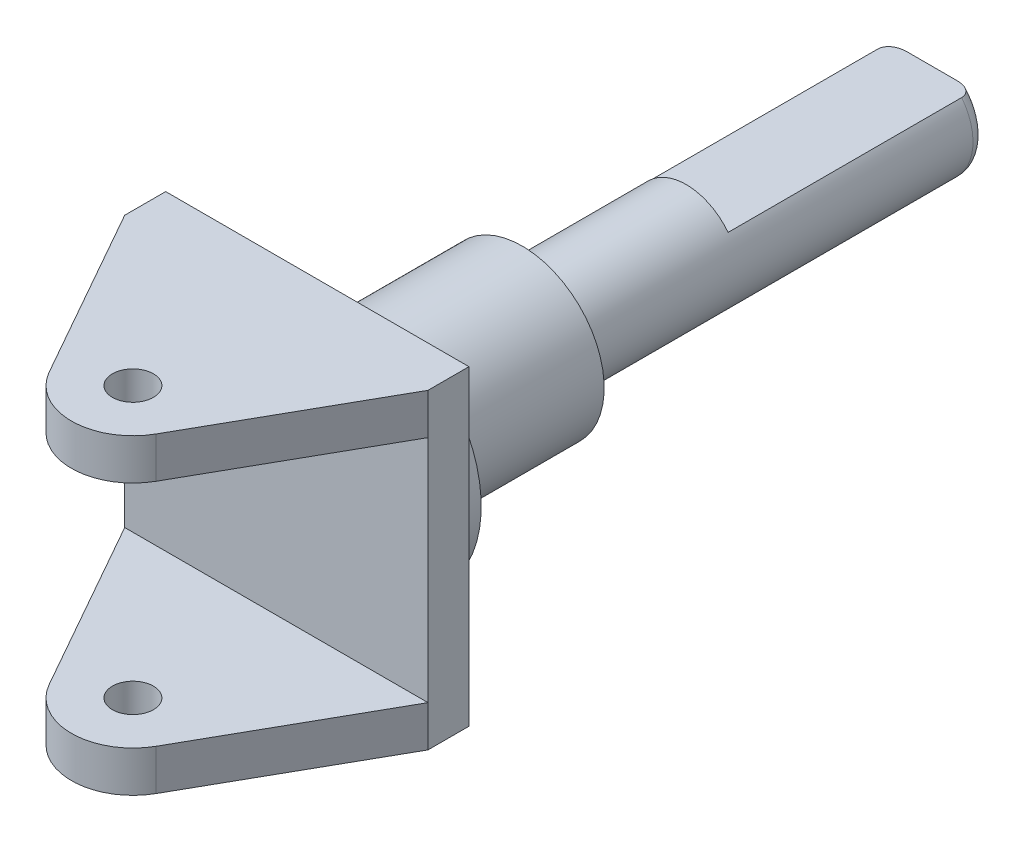
ISO-10303-21;
HEADER;
FILE_DESCRIPTION(('STEP AP214'),'2;1');
FILE_NAME('part.step','',(''),(''),'','','');
FILE_SCHEMA(('AUTOMOTIVE_DESIGN { 1 0 10303 214 1 1 1 1 }'));
ENDSEC;
DATA;
#1=APPLICATION_CONTEXT('core data for automotive mechanical design processes');
#2=APPLICATION_PROTOCOL_DEFINITION('international standard','automotive_design',2000,#1);
#3=PRODUCT_CONTEXT('',#1,'mechanical');
#4=PRODUCT('Part','Part','',(#3));
#5=PRODUCT_RELATED_PRODUCT_CATEGORY('part','',(#4));
#6=PRODUCT_DEFINITION_FORMATION('','',#4);
#7=PRODUCT_DEFINITION_CONTEXT('part definition',#1,'design');
#8=PRODUCT_DEFINITION('design','',#6,#7);
#9=PRODUCT_DEFINITION_SHAPE('','',#8);
#10=(LENGTH_UNIT() NAMED_UNIT(*) SI_UNIT(.MILLI.,.METRE.));
#11=(NAMED_UNIT(*) PLANE_ANGLE_UNIT() SI_UNIT($,.RADIAN.));
#12=(NAMED_UNIT(*) SI_UNIT($,.STERADIAN.) SOLID_ANGLE_UNIT());
#13=UNCERTAINTY_MEASURE_WITH_UNIT(LENGTH_MEASURE(1.E-05),#10,'distance_accuracy_value','');
#14=(GEOMETRIC_REPRESENTATION_CONTEXT(3) GLOBAL_UNCERTAINTY_ASSIGNED_CONTEXT((#13)) GLOBAL_UNIT_ASSIGNED_CONTEXT((#10,
#11,#12)) REPRESENTATION_CONTEXT('',''));
#15=CARTESIAN_POINT('',(0.,0.,0.));
#16=DIRECTION('',(0.,0.,1.));
#17=DIRECTION('',(1.,0.,0.));
#18=AXIS2_PLACEMENT_3D('',#15,#16,#17);
#19=CARTESIAN_POINT('',(0.,0.,10.));
#20=DIRECTION('',(0.,0.,-1.));
#21=DIRECTION('',(-1.,0.,0.));
#22=AXIS2_PLACEMENT_3D('',#19,#20,#21);
#23=PLANE('',#22);
#24=DIRECTION('',(0.,-1.,0.));
#25=VECTOR('',#24,1.);
#26=CARTESIAN_POINT('',(-37.,-38.,10.));
#27=LINE('',#26,#25);
#28=CARTESIAN_POINT('',(-37.,28.,10.));
#29=VERTEX_POINT('',#28);
#30=CARTESIAN_POINT('',(-37.,-28.,10.));
#31=VERTEX_POINT('',#30);
#32=EDGE_CURVE('E290',#29,#31,#27,.T.);
#33=ORIENTED_EDGE('',*,*,#32,.T.);
#34=DIRECTION('',(1.,0.,0.));
#35=VECTOR('',#34,1.);
#36=CARTESIAN_POINT('',(-37.,-28.,10.));
#37=LINE('',#36,#35);
#38=CARTESIAN_POINT('',(37.,-28.,10.));
#39=VERTEX_POINT('',#38);
#40=EDGE_CURVE('E224',#31,#39,#37,.T.);
#41=ORIENTED_EDGE('',*,*,#40,.T.);
#42=DIRECTION('',(0.,1.,0.));
#43=VECTOR('',#42,1.);
#44=CARTESIAN_POINT('',(37.,-38.,10.));
#45=LINE('',#44,#43);
#46=CARTESIAN_POINT('',(37.,28.,10.));
#47=VERTEX_POINT('',#46);
#48=EDGE_CURVE('E288',#39,#47,#45,.T.);
#49=ORIENTED_EDGE('',*,*,#48,.T.);
#50=DIRECTION('',(1.,0.,0.));
#51=VECTOR('',#50,1.);
#52=CARTESIAN_POINT('',(0.,28.,10.));
#53=LINE('',#52,#51);
#54=EDGE_CURVE('E263',#29,#47,#53,.T.);
#55=ORIENTED_EDGE('',*,*,#54,.F.);
#56=EDGE_LOOP('',(#33,#41,#49,#55));
#57=FACE_BOUND('',#56,.T.);
#58=ADVANCED_FACE('F41',(#57),#23,.F.);
#59=CARTESIAN_POINT('',(37.,-38.,10.));
#60=DIRECTION('',(-1.,0.,0.));
#61=DIRECTION('',(0.,0.,1.));
#62=AXIS2_PLACEMENT_3D('',#59,#60,#61);
#63=PLANE('',#62);
#64=DIRECTION('',(0.,1.,0.));
#65=VECTOR('',#64,1.);
#66=CARTESIAN_POINT('',(37.,-38.,0.));
#67=LINE('',#66,#65);
#68=CARTESIAN_POINT('',(37.,-38.,0.));
#69=VERTEX_POINT('',#68);
#70=CARTESIAN_POINT('',(37.,38.,0.));
#71=VERTEX_POINT('',#70);
#72=EDGE_CURVE('E278',#69,#71,#67,.T.);
#73=ORIENTED_EDGE('',*,*,#72,.T.);
#74=DIRECTION('',(0.,0.,-1.));
#75=VECTOR('',#74,1.);
#76=CARTESIAN_POINT('',(37.,38.,10.));
#77=LINE('',#76,#75);
#78=CARTESIAN_POINT('',(37.,38.,10.));
#79=VERTEX_POINT('',#78);
#80=EDGE_CURVE('E190',#79,#71,#77,.T.);
#81=ORIENTED_EDGE('',*,*,#80,.F.);
#82=DIRECTION('',(0.,1.,0.));
#83=VECTOR('',#82,1.);
#84=CARTESIAN_POINT('',(37.,28.,10.));
#85=LINE('',#84,#83);
#86=EDGE_CURVE('E280',#47,#79,#85,.T.);
#87=ORIENTED_EDGE('',*,*,#86,.F.);
#88=ORIENTED_EDGE('',*,*,#48,.F.);
#89=CARTESIAN_POINT('',(37.,-38.,10.));
#90=VERTEX_POINT('',#89);
#91=EDGE_CURVE('E282',#90,#39,#45,.T.);
#92=ORIENTED_EDGE('',*,*,#91,.F.);
#93=DIRECTION('',(0.,0.,-1.));
#94=VECTOR('',#93,1.);
#95=CARTESIAN_POINT('',(37.,-38.,10.));
#96=LINE('',#95,#94);
#97=EDGE_CURVE('E295',#90,#69,#96,.T.);
#98=ORIENTED_EDGE('',*,*,#97,.T.);
#99=EDGE_LOOP('',(#73,#81,#87,#88,#92,#98));
#100=FACE_BOUND('',#99,.T.);
#101=ADVANCED_FACE('F403',(#100),#63,.F.);
#102=CARTESIAN_POINT('',(-37.,38.,10.));
#103=DIRECTION('',(0.,-1.,0.));
#104=DIRECTION('',(0.,0.,-1.));
#105=AXIS2_PLACEMENT_3D('',#102,#103,#104);
#106=PLANE('',#105);
#107=DIRECTION('',(-1.,0.,0.));
#108=VECTOR('',#107,1.);
#109=CARTESIAN_POINT('',(-37.,38.,0.));
#110=LINE('',#109,#108);
#111=CARTESIAN_POINT('',(-37.,38.,0.));
#112=VERTEX_POINT('',#111);
#113=EDGE_CURVE('E293',#71,#112,#110,.T.);
#114=ORIENTED_EDGE('',*,*,#113,.T.);
#115=DIRECTION('',(0.,0.,-1.));
#116=VECTOR('',#115,1.);
#117=CARTESIAN_POINT('',(-37.,38.,10.));
#118=LINE('',#117,#116);
#119=CARTESIAN_POINT('',(-37.,38.,10.));
#120=VERTEX_POINT('',#119);
#121=EDGE_CURVE('E308',#120,#112,#118,.T.);
#122=ORIENTED_EDGE('',*,*,#121,.F.);
#123=DIRECTION('',(0.491857302042567,0.,0.870675826256482));
#124=VECTOR('',#123,1.);
#125=CARTESIAN_POINT('',(-32.331309222376,38.,18.2644217814052));
#126=LINE('',#125,#124);
#127=CARTESIAN_POINT('',(-13.0601373938472,38.,52.3778595306385));
#128=VERTEX_POINT('',#127);
#129=EDGE_CURVE('E267',#120,#128,#126,.T.);
#130=ORIENTED_EDGE('',*,*,#129,.T.);
#131=CARTESIAN_POINT('',(0.,38.,45.));
#132=DIRECTION('',(0.,1.,0.));
#133=DIRECTION('',(0.,0.,1.));
#134=AXIS2_PLACEMENT_3D('',#131,#132,#133);
#135=CIRCLE('',#134,15.);
#136=CARTESIAN_POINT('',(13.0601373938472,38.,52.3778595306385));
#137=VERTEX_POINT('',#136);
#138=EDGE_CURVE('E275',#128,#137,#135,.T.);
#139=ORIENTED_EDGE('',*,*,#138,.T.);
#140=DIRECTION('',(0.491857302042567,0.,-0.870675826256482));
#141=VECTOR('',#140,1.);
#142=CARTESIAN_POINT('',(32.331309222376,38.,18.2644217814052));
#143=LINE('',#142,#141);
#144=EDGE_CURVE('E255',#137,#79,#143,.T.);
#145=ORIENTED_EDGE('',*,*,#144,.T.);
#146=ORIENTED_EDGE('',*,*,#80,.T.);
#147=EDGE_LOOP('',(#114,#122,#130,#139,#145,#146));
#148=FACE_BOUND('',#147,.T.);
#149=CARTESIAN_POINT('',(0.,38.,45.));
#150=DIRECTION('',(0.,1.,0.));
#151=DIRECTION('',(0.,0.,1.));
#152=AXIS2_PLACEMENT_3D('',#149,#150,#151);
#153=CIRCLE('',#152,5.);
#154=CARTESIAN_POINT('',(0.,38.,50.));
#155=VERTEX_POINT('',#154);
#156=EDGE_CURVE('E247',#155,#155,#153,.T.);
#157=ORIENTED_EDGE('',*,*,#156,.F.);
#158=EDGE_LOOP('',(#157));
#159=FACE_BOUND('',#158,.T.);
#160=ADVANCED_FACE('F417',(#148,#159),#106,.F.);
#161=CARTESIAN_POINT('',(-37.,-38.,10.));
#162=DIRECTION('',(1.,0.,0.));
#163=DIRECTION('',(0.,0.,-1.));
#164=AXIS2_PLACEMENT_3D('',#161,#162,#163);
#165=PLANE('',#164);
#166=DIRECTION('',(0.,-1.,0.));
#167=VECTOR('',#166,1.);
#168=CARTESIAN_POINT('',(-37.,-38.,0.));
#169=LINE('',#168,#167);
#170=CARTESIAN_POINT('',(-37.,-38.,0.));
#171=VERTEX_POINT('',#170);
#172=EDGE_CURVE('E300',#112,#171,#169,.T.);
#173=ORIENTED_EDGE('',*,*,#172,.T.);
#174=DIRECTION('',(0.,0.,-1.));
#175=VECTOR('',#174,1.);
#176=CARTESIAN_POINT('',(-37.,-38.,10.));
#177=LINE('',#176,#175);
#178=CARTESIAN_POINT('',(-37.,-38.,10.));
#179=VERTEX_POINT('',#178);
#180=EDGE_CURVE('E303',#179,#171,#177,.T.);
#181=ORIENTED_EDGE('',*,*,#180,.F.);
#182=DIRECTION('',(0.,-1.,0.));
#183=VECTOR('',#182,1.);
#184=CARTESIAN_POINT('',(-37.,-28.,10.));
#185=LINE('',#184,#183);
#186=EDGE_CURVE('E241',#31,#179,#185,.T.);
#187=ORIENTED_EDGE('',*,*,#186,.F.);
#188=ORIENTED_EDGE('',*,*,#32,.F.);
#189=EDGE_CURVE('E289',#120,#29,#27,.T.);
#190=ORIENTED_EDGE('',*,*,#189,.F.);
#191=ORIENTED_EDGE('',*,*,#121,.T.);
#192=EDGE_LOOP('',(#173,#181,#187,#188,#190,#191));
#193=FACE_BOUND('',#192,.T.);
#194=ADVANCED_FACE('F413',(#193),#165,.F.);
#195=CARTESIAN_POINT('',(-37.,-38.,10.));
#196=DIRECTION('',(0.,1.,0.));
#197=DIRECTION('',(0.,0.,1.));
#198=AXIS2_PLACEMENT_3D('',#195,#196,#197);
#199=PLANE('',#198);
#200=DIRECTION('',(1.,0.,0.));
#201=VECTOR('',#200,1.);
#202=CARTESIAN_POINT('',(-37.,-38.,0.));
#203=LINE('',#202,#201);
#204=EDGE_CURVE('E297',#171,#69,#203,.T.);
#205=ORIENTED_EDGE('',*,*,#204,.T.);
#206=ORIENTED_EDGE('',*,*,#97,.F.);
#207=DIRECTION('',(-0.491857302042567,0.,0.870675826256482));
#208=VECTOR('',#207,1.);
#209=CARTESIAN_POINT('',(37.,-38.,10.));
#210=LINE('',#209,#208);
#211=CARTESIAN_POINT('',(13.0601373938472,-38.,52.3778595306385));
#212=VERTEX_POINT('',#211);
#213=EDGE_CURVE('E219',#90,#212,#210,.T.);
#214=ORIENTED_EDGE('',*,*,#213,.T.);
#215=CARTESIAN_POINT('',(0.,-38.,44.9999999999996));
#216=DIRECTION('',(0.,-1.,0.));
#217=DIRECTION('',(0.,0.,1.));
#218=AXIS2_PLACEMENT_3D('',#215,#216,#217);
#219=CIRCLE('',#218,15.0000000000002);
#220=CARTESIAN_POINT('',(-13.0601373938472,-38.,52.3778595306385));
#221=VERTEX_POINT('',#220);
#222=EDGE_CURVE('E236',#212,#221,#219,.T.);
#223=ORIENTED_EDGE('',*,*,#222,.T.);
#224=DIRECTION('',(-0.491857302042567,0.,-0.870675826256482));
#225=VECTOR('',#224,1.);
#226=CARTESIAN_POINT('',(-37.,-38.,10.));
#227=LINE('',#226,#225);
#228=EDGE_CURVE('E228',#221,#179,#227,.T.);
#229=ORIENTED_EDGE('',*,*,#228,.T.);
#230=ORIENTED_EDGE('',*,*,#180,.T.);
#231=EDGE_LOOP('',(#205,#206,#214,#223,#229,#230));
#232=FACE_BOUND('',#231,.T.);
#233=CARTESIAN_POINT('',(0.,-38.,44.9999999999996));
#234=DIRECTION('',(0.,-1.,0.));
#235=DIRECTION('',(0.,0.,-1.));
#236=AXIS2_PLACEMENT_3D('',#233,#234,#235);
#237=CIRCLE('',#236,4.9999999999998);
#238=CARTESIAN_POINT('',(0.,-38.,39.9999999999998));
#239=VERTEX_POINT('',#238);
#240=EDGE_CURVE('E216',#239,#239,#237,.T.);
#241=ORIENTED_EDGE('',*,*,#240,.F.);
#242=EDGE_LOOP('',(#241));
#243=FACE_BOUND('',#242,.T.);
#244=ADVANCED_FACE('F407',(#232,#243),#199,.F.);
#245=CARTESIAN_POINT('',(0.,0.,0.));
#246=DIRECTION('',(0.,0.,-1.));
#247=DIRECTION('',(-1.,0.,0.));
#248=AXIS2_PLACEMENT_3D('',#245,#246,#247);
#249=PLANE('',#248);
#250=CARTESIAN_POINT('',(0.,0.,0.));
#251=DIRECTION('',(0.,0.,-1.));
#252=DIRECTION('',(-1.,0.,0.));
#253=AXIS2_PLACEMENT_3D('',#250,#251,#252);
#254=CIRCLE('',#253,30.);
#255=CARTESIAN_POINT('',(-19.9214744270855,-22.4306677709555,0.));
#256=VERTEX_POINT('',#255);
#257=CARTESIAN_POINT('',(-19.9214744270848,22.430667770956,0.));
#258=VERTEX_POINT('',#257);
#259=EDGE_CURVE('E184',#256,#258,#254,.T.);
#260=ORIENTED_EDGE('',*,*,#259,.F.);
#261=DIRECTION('',(-0.999883722331186,-0.0152493218580814,0.));
#262=VECTOR('',#261,1.);
#263=CARTESIAN_POINT('',(0.337380123403688,-22.1216980511602,0.));
#264=LINE('',#263,#262);
#265=CARTESIAN_POINT('',(20.5962346738928,-21.812728331365,0.));
#266=VERTEX_POINT('',#265);
#267=EDGE_CURVE('E192',#266,#256,#264,.T.);
#268=ORIENTED_EDGE('',*,*,#267,.F.);
#269=CARTESIAN_POINT('',(0.,0.,0.));
#270=DIRECTION('',(0.,0.,-1.));
#271=DIRECTION('',(-1.,0.,0.));
#272=AXIS2_PLACEMENT_3D('',#269,#270,#271);
#273=CIRCLE('',#272,30.);
#274=CARTESIAN_POINT('',(20.5962346738934,21.8127283313644,0.));
#275=VERTEX_POINT('',#274);
#276=EDGE_CURVE('E201',#275,#266,#273,.T.);
#277=ORIENTED_EDGE('',*,*,#276,.F.);
#278=DIRECTION('',(-0.999883722331186,0.0152493218581099,0.));
#279=VECTOR('',#278,1.);
#280=CARTESIAN_POINT('',(0.337380123404318,22.1216980511602,0.));
#281=LINE('',#280,#279);
#282=EDGE_CURVE('E199',#275,#258,#281,.T.);
#283=ORIENTED_EDGE('',*,*,#282,.T.);
#284=EDGE_LOOP('',(#260,#268,#277,#283));
#285=FACE_BOUND('',#284,.T.);
#286=ORIENTED_EDGE('',*,*,#72,.F.);
#287=ORIENTED_EDGE('',*,*,#204,.F.);
#288=ORIENTED_EDGE('',*,*,#172,.F.);
#289=ORIENTED_EDGE('',*,*,#113,.F.);
#290=EDGE_LOOP('',(#286,#287,#288,#289));
#291=FACE_BOUND('',#290,.T.);
#292=ADVANCED_FACE('F398',(#285,#291),#249,.T.);
#293=CARTESIAN_POINT('',(-32.331309222376,28.,18.2644217814052));
#294=DIRECTION('',(-0.870675826256482,0.,0.491857302042566));
#295=DIRECTION('',(0.491857302042566,0.,0.870675826256482));
#296=AXIS2_PLACEMENT_3D('',#293,#294,#295);
#297=PLANE('',#296);
#298=ORIENTED_EDGE('',*,*,#129,.F.);
#299=ORIENTED_EDGE('',*,*,#189,.T.);
#300=DIRECTION('',(0.491857302042567,0.,0.870675826256482));
#301=VECTOR('',#300,1.);
#302=CARTESIAN_POINT('',(-32.331309222376,28.,18.2644217814052));
#303=LINE('',#302,#301);
#304=CARTESIAN_POINT('',(-13.0601373938472,28.,52.3778595306385));
#305=VERTEX_POINT('',#304);
#306=EDGE_CURVE('E251',#29,#305,#303,.T.);
#307=ORIENTED_EDGE('',*,*,#306,.T.);
#308=DIRECTION('',(0.,1.,0.));
#309=VECTOR('',#308,1.);
#310=CARTESIAN_POINT('',(-13.0601373938472,28.,52.3778595306385));
#311=LINE('',#310,#309);
#312=EDGE_CURVE('E266',#305,#128,#311,.T.);
#313=ORIENTED_EDGE('',*,*,#312,.T.);
#314=EDGE_LOOP('',(#298,#299,#307,#313));
#315=FACE_BOUND('',#314,.T.);
#316=ADVANCED_FACE('F393',(#315),#297,.T.);
#317=CARTESIAN_POINT('',(32.331309222376,28.,18.2644217814052));
#318=DIRECTION('',(0.870675826256482,0.,0.491857302042567));
#319=DIRECTION('',(0.491857302042567,0.,-0.870675826256482));
#320=AXIS2_PLACEMENT_3D('',#317,#318,#319);
#321=PLANE('',#320);
#322=ORIENTED_EDGE('',*,*,#144,.F.);
#323=DIRECTION('',(0.,1.,0.));
#324=VECTOR('',#323,1.);
#325=CARTESIAN_POINT('',(13.0601373938472,28.,52.3778595306385));
#326=LINE('',#325,#324);
#327=CARTESIAN_POINT('',(13.0601373938472,28.,52.3778595306385));
#328=VERTEX_POINT('',#327);
#329=EDGE_CURVE('E283',#328,#137,#326,.T.);
#330=ORIENTED_EDGE('',*,*,#329,.F.);
#331=DIRECTION('',(0.491857302042567,0.,-0.870675826256482));
#332=VECTOR('',#331,1.);
#333=CARTESIAN_POINT('',(32.331309222376,28.,18.2644217814052));
#334=LINE('',#333,#332);
#335=EDGE_CURVE('E257',#328,#47,#334,.T.);
#336=ORIENTED_EDGE('',*,*,#335,.T.);
#337=ORIENTED_EDGE('',*,*,#86,.T.);
#338=EDGE_LOOP('',(#322,#330,#336,#337));
#339=FACE_BOUND('',#338,.T.);
#340=ADVANCED_FACE('F390',(#339),#321,.T.);
#341=CARTESIAN_POINT('',(0.,28.,45.));
#342=DIRECTION('',(0.,1.,0.));
#343=DIRECTION('',(0.,0.,1.));
#344=AXIS2_PLACEMENT_3D('',#341,#342,#343);
#345=CYLINDRICAL_SURFACE('',#344,5.);
#346=CARTESIAN_POINT('',(0.,28.,45.));
#347=DIRECTION('',(0.,1.,0.));
#348=DIRECTION('',(0.,0.,1.));
#349=AXIS2_PLACEMENT_3D('',#346,#347,#348);
#350=CIRCLE('',#349,5.);
#351=CARTESIAN_POINT('',(0.,28.,50.));
#352=VERTEX_POINT('',#351);
#353=EDGE_CURVE('E246',#352,#352,#350,.T.);
#354=ORIENTED_EDGE('',*,*,#353,.F.);
#355=EDGE_LOOP('',(#354));
#356=FACE_BOUND('',#355,.T.);
#357=ORIENTED_EDGE('',*,*,#156,.T.);
#358=EDGE_LOOP('',(#357));
#359=FACE_BOUND('',#358,.T.);
#360=ADVANCED_FACE('F388',(#356,#359),#345,.F.);
#361=CARTESIAN_POINT('',(0.,28.,45.));
#362=DIRECTION('',(0.,1.,0.));
#363=DIRECTION('',(0.,0.,1.));
#364=AXIS2_PLACEMENT_3D('',#361,#362,#363);
#365=CYLINDRICAL_SURFACE('',#364,15.);
#366=ORIENTED_EDGE('',*,*,#138,.F.);
#367=ORIENTED_EDGE('',*,*,#312,.F.);
#368=CARTESIAN_POINT('',(0.,28.,45.));
#369=DIRECTION('',(0.,1.,0.));
#370=DIRECTION('',(0.,0.,1.));
#371=AXIS2_PLACEMENT_3D('',#368,#369,#370);
#372=CIRCLE('',#371,15.);
#373=EDGE_CURVE('E260',#305,#328,#372,.T.);
#374=ORIENTED_EDGE('',*,*,#373,.T.);
#375=ORIENTED_EDGE('',*,*,#329,.T.);
#376=EDGE_LOOP('',(#366,#367,#374,#375));
#377=FACE_BOUND('',#376,.T.);
#378=ADVANCED_FACE('F384',(#377),#365,.T.);
#379=CARTESIAN_POINT('',(0.,28.,0.));
#380=DIRECTION('',(0.,1.,0.));
#381=DIRECTION('',(0.,0.,1.));
#382=AXIS2_PLACEMENT_3D('',#379,#380,#381);
#383=PLANE('',#382);
#384=ORIENTED_EDGE('',*,*,#353,.T.);
#385=EDGE_LOOP('',(#384));
#386=FACE_BOUND('',#385,.T.);
#387=ORIENTED_EDGE('',*,*,#306,.F.);
#388=ORIENTED_EDGE('',*,*,#54,.T.);
#389=ORIENTED_EDGE('',*,*,#335,.F.);
#390=ORIENTED_EDGE('',*,*,#373,.F.);
#391=EDGE_LOOP('',(#387,#388,#389,#390));
#392=FACE_BOUND('',#391,.T.);
#393=ADVANCED_FACE('F374',(#386,#392),#383,.F.);
#394=CARTESIAN_POINT('',(-37.,-28.,10.));
#395=DIRECTION('',(-0.870675826256482,0.,0.491857302042567));
#396=DIRECTION('',(0.491857302042567,0.,0.870675826256482));
#397=AXIS2_PLACEMENT_3D('',#394,#395,#396);
#398=PLANE('',#397);
#399=ORIENTED_EDGE('',*,*,#228,.F.);
#400=DIRECTION('',(0.,-1.,0.));
#401=VECTOR('',#400,1.);
#402=CARTESIAN_POINT('',(-13.0601373938472,-28.,52.3778595306385));
#403=LINE('',#402,#401);
#404=CARTESIAN_POINT('',(-13.0601373938472,-28.,52.3778595306385));
#405=VERTEX_POINT('',#404);
#406=EDGE_CURVE('E250',#405,#221,#403,.T.);
#407=ORIENTED_EDGE('',*,*,#406,.F.);
#408=DIRECTION('',(-0.491857302042567,0.,-0.870675826256482));
#409=VECTOR('',#408,1.);
#410=CARTESIAN_POINT('',(-37.,-28.,10.));
#411=LINE('',#410,#409);
#412=EDGE_CURVE('E235',#405,#31,#411,.T.);
#413=ORIENTED_EDGE('',*,*,#412,.T.);
#414=ORIENTED_EDGE('',*,*,#186,.T.);
#415=EDGE_LOOP('',(#399,#407,#413,#414));
#416=FACE_BOUND('',#415,.T.);
#417=ADVANCED_FACE('F371',(#416),#398,.T.);
#418=CARTESIAN_POINT('',(0.,-28.,44.9999999999996));
#419=DIRECTION('',(0.,-1.,0.));
#420=DIRECTION('',(0.,0.,-1.));
#421=AXIS2_PLACEMENT_3D('',#418,#419,#420);
#422=CYLINDRICAL_SURFACE('',#421,15.0000000000002);
#423=ORIENTED_EDGE('',*,*,#222,.F.);
#424=DIRECTION('',(0.,-1.,0.));
#425=VECTOR('',#424,1.);
#426=CARTESIAN_POINT('',(13.0601373938472,-28.,52.3778595306385));
#427=LINE('',#426,#425);
#428=CARTESIAN_POINT('',(13.0601373938472,-28.,52.3778595306385));
#429=VERTEX_POINT('',#428);
#430=EDGE_CURVE('E231',#429,#212,#427,.T.);
#431=ORIENTED_EDGE('',*,*,#430,.F.);
#432=CARTESIAN_POINT('',(0.,-28.,44.9999999999996));
#433=DIRECTION('',(0.,-1.,0.));
#434=DIRECTION('',(0.,0.,1.));
#435=AXIS2_PLACEMENT_3D('',#432,#433,#434);
#436=CIRCLE('',#435,15.0000000000002);
#437=EDGE_CURVE('E227',#429,#405,#436,.T.);
#438=ORIENTED_EDGE('',*,*,#437,.T.);
#439=ORIENTED_EDGE('',*,*,#406,.T.);
#440=EDGE_LOOP('',(#423,#431,#438,#439));
#441=FACE_BOUND('',#440,.T.);
#442=ADVANCED_FACE('F372',(#441),#422,.T.);
#443=CARTESIAN_POINT('',(37.,-28.,10.));
#444=DIRECTION('',(0.870675826256482,0.,0.491857302042566));
#445=DIRECTION('',(0.491857302042566,0.,-0.870675826256482));
#446=AXIS2_PLACEMENT_3D('',#443,#444,#445);
#447=PLANE('',#446);
#448=ORIENTED_EDGE('',*,*,#213,.F.);
#449=ORIENTED_EDGE('',*,*,#91,.T.);
#450=DIRECTION('',(-0.491857302042567,0.,0.870675826256482));
#451=VECTOR('',#450,1.);
#452=CARTESIAN_POINT('',(37.,-28.,10.));
#453=LINE('',#452,#451);
#454=EDGE_CURVE('E223',#39,#429,#453,.T.);
#455=ORIENTED_EDGE('',*,*,#454,.T.);
#456=ORIENTED_EDGE('',*,*,#430,.T.);
#457=EDGE_LOOP('',(#448,#449,#455,#456));
#458=FACE_BOUND('',#457,.T.);
#459=ADVANCED_FACE('F369',(#458),#447,.T.);
#460=CARTESIAN_POINT('',(0.,-28.,44.9999999999996));
#461=DIRECTION('',(0.,1.,0.));
#462=DIRECTION('',(0.,0.,1.));
#463=AXIS2_PLACEMENT_3D('',#460,#461,#462);
#464=PLANE('',#463);
#465=CARTESIAN_POINT('',(0.,-28.,44.9999999999996));
#466=DIRECTION('',(0.,-1.,0.));
#467=DIRECTION('',(0.,0.,-1.));
#468=AXIS2_PLACEMENT_3D('',#465,#466,#467);
#469=CIRCLE('',#468,4.9999999999998);
#470=CARTESIAN_POINT('',(0.,-28.,39.9999999999998));
#471=VERTEX_POINT('',#470);
#472=EDGE_CURVE('E220',#471,#471,#469,.T.);
#473=ORIENTED_EDGE('',*,*,#472,.T.);
#474=EDGE_LOOP('',(#473));
#475=FACE_BOUND('',#474,.T.);
#476=ORIENTED_EDGE('',*,*,#40,.F.);
#477=ORIENTED_EDGE('',*,*,#412,.F.);
#478=ORIENTED_EDGE('',*,*,#437,.F.);
#479=ORIENTED_EDGE('',*,*,#454,.F.);
#480=EDGE_LOOP('',(#476,#477,#478,#479));
#481=FACE_BOUND('',#480,.T.);
#482=ADVANCED_FACE('F364',(#475,#481),#464,.T.);
#483=CARTESIAN_POINT('',(0.,-28.,44.9999999999996));
#484=DIRECTION('',(0.,-1.,0.));
#485=DIRECTION('',(0.,0.,-1.));
#486=AXIS2_PLACEMENT_3D('',#483,#484,#485);
#487=CYLINDRICAL_SURFACE('',#486,4.9999999999998);
#488=ORIENTED_EDGE('',*,*,#472,.F.);
#489=EDGE_LOOP('',(#488));
#490=FACE_BOUND('',#489,.T.);
#491=ORIENTED_EDGE('',*,*,#240,.T.);
#492=EDGE_LOOP('',(#491));
#493=FACE_BOUND('',#492,.T.);
#494=ADVANCED_FACE('F363',(#490,#493),#487,.F.);
#495=CARTESIAN_POINT('',(0.,0.,-10.));
#496=DIRECTION('',(0.,0.,1.));
#497=DIRECTION('',(1.,0.,0.));
#498=AXIS2_PLACEMENT_3D('',#495,#496,#497);
#499=CYLINDRICAL_SURFACE('',#498,30.);
#500=ORIENTED_EDGE('',*,*,#259,.T.);
#501=DIRECTION('',(0.,0.,1.));
#502=VECTOR('',#501,1.);
#503=CARTESIAN_POINT('',(-19.9214744270848,22.430667770956,-10.));
#504=LINE('',#503,#502);
#505=CARTESIAN_POINT('',(-19.9214744270848,22.430667770956,-10.));
#506=VERTEX_POINT('',#505);
#507=EDGE_CURVE('E213',#506,#258,#504,.T.);
#508=ORIENTED_EDGE('',*,*,#507,.F.);
#509=CARTESIAN_POINT('',(0.,0.,-10.));
#510=DIRECTION('',(0.,0.,-1.));
#511=DIRECTION('',(-1.,0.,0.));
#512=AXIS2_PLACEMENT_3D('',#509,#510,#511);
#513=CIRCLE('',#512,30.);
#514=CARTESIAN_POINT('',(-19.9214744270855,-22.4306677709555,-10.));
#515=VERTEX_POINT('',#514);
#516=EDGE_CURVE('E186',#515,#506,#513,.T.);
#517=ORIENTED_EDGE('',*,*,#516,.F.);
#518=DIRECTION('',(0.,0.,1.));
#519=VECTOR('',#518,1.);
#520=CARTESIAN_POINT('',(-19.9214744270855,-22.4306677709555,-10.));
#521=LINE('',#520,#519);
#522=EDGE_CURVE('E196',#515,#256,#521,.T.);
#523=ORIENTED_EDGE('',*,*,#522,.T.);
#524=EDGE_LOOP('',(#500,#508,#517,#523));
#525=FACE_BOUND('',#524,.T.);
#526=ADVANCED_FACE('F360',(#525),#499,.T.);
#527=CARTESIAN_POINT('',(0.337380123404318,22.1216980511602,-10.));
#528=DIRECTION('',(0.0152493218581099,0.999883722331186,0.));
#529=DIRECTION('',(-0.999883722331186,0.0152493218581099,0.));
#530=AXIS2_PLACEMENT_3D('',#527,#528,#529);
#531=PLANE('',#530);
#532=ORIENTED_EDGE('',*,*,#282,.F.);
#533=DIRECTION('',(0.,0.,1.));
#534=VECTOR('',#533,1.);
#535=CARTESIAN_POINT('',(20.5962346738934,21.8127283313644,-10.));
#536=LINE('',#535,#534);
#537=CARTESIAN_POINT('',(20.5962346738934,21.8127283313644,-10.));
#538=VERTEX_POINT('',#537);
#539=EDGE_CURVE('E211',#538,#275,#536,.T.);
#540=ORIENTED_EDGE('',*,*,#539,.F.);
#541=DIRECTION('',(-0.999883722331186,0.0152493218581099,0.));
#542=VECTOR('',#541,1.);
#543=CARTESIAN_POINT('',(0.337380123404318,22.1216980511602,-10.));
#544=LINE('',#543,#542);
#545=EDGE_CURVE('E189',#538,#506,#544,.T.);
#546=ORIENTED_EDGE('',*,*,#545,.T.);
#547=ORIENTED_EDGE('',*,*,#507,.T.);
#548=EDGE_LOOP('',(#532,#540,#546,#547));
#549=FACE_BOUND('',#548,.T.);
#550=ADVANCED_FACE('F351',(#549),#531,.T.);
#551=CARTESIAN_POINT('',(0.,0.,-10.));
#552=DIRECTION('',(0.,0.,1.));
#553=DIRECTION('',(1.,0.,0.));
#554=AXIS2_PLACEMENT_3D('',#551,#552,#553);
#555=CYLINDRICAL_SURFACE('',#554,30.);
#556=ORIENTED_EDGE('',*,*,#276,.T.);
#557=DIRECTION('',(0.,0.,1.));
#558=VECTOR('',#557,1.);
#559=CARTESIAN_POINT('',(20.5962346738928,-21.812728331365,-10.));
#560=LINE('',#559,#558);
#561=CARTESIAN_POINT('',(20.5962346738928,-21.812728331365,-10.));
#562=VERTEX_POINT('',#561);
#563=EDGE_CURVE('E208',#562,#266,#560,.T.);
#564=ORIENTED_EDGE('',*,*,#563,.F.);
#565=CARTESIAN_POINT('',(0.,0.,-10.));
#566=DIRECTION('',(0.,0.,-1.));
#567=DIRECTION('',(-1.,0.,0.));
#568=AXIS2_PLACEMENT_3D('',#565,#566,#567);
#569=CIRCLE('',#568,30.);
#570=EDGE_CURVE('E194',#538,#562,#569,.T.);
#571=ORIENTED_EDGE('',*,*,#570,.F.);
#572=ORIENTED_EDGE('',*,*,#539,.T.);
#573=EDGE_LOOP('',(#556,#564,#571,#572));
#574=FACE_BOUND('',#573,.T.);
#575=ADVANCED_FACE('F349',(#574),#555,.T.);
#576=CARTESIAN_POINT('',(0.337380123403688,-22.1216980511602,-10.));
#577=DIRECTION('',(-0.0152493218580814,0.999883722331186,0.));
#578=DIRECTION('',(-0.999883722331186,-0.0152493218580814,0.));
#579=AXIS2_PLACEMENT_3D('',#576,#577,#578);
#580=PLANE('',#579);
#581=ORIENTED_EDGE('',*,*,#267,.T.);
#582=ORIENTED_EDGE('',*,*,#522,.F.);
#583=DIRECTION('',(-0.999883722331186,-0.0152493218580814,0.));
#584=VECTOR('',#583,1.);
#585=CARTESIAN_POINT('',(0.337380123403688,-22.1216980511602,-10.));
#586=LINE('',#585,#584);
#587=EDGE_CURVE('E198',#562,#515,#586,.T.);
#588=ORIENTED_EDGE('',*,*,#587,.F.);
#589=ORIENTED_EDGE('',*,*,#563,.T.);
#590=EDGE_LOOP('',(#581,#582,#588,#589));
#591=FACE_BOUND('',#590,.T.);
#592=ADVANCED_FACE('F341',(#591),#580,.F.);
#593=CARTESIAN_POINT('',(0.,0.,-10.));
#594=DIRECTION('',(0.,0.,-1.));
#595=DIRECTION('',(-1.,0.,0.));
#596=AXIS2_PLACEMENT_3D('',#593,#594,#595);
#597=PLANE('',#596);
#598=CARTESIAN_POINT('',(0.,0.,-10.));
#599=DIRECTION('',(0.,0.,-1.));
#600=DIRECTION('',(-1.,0.,0.));
#601=AXIS2_PLACEMENT_3D('',#598,#599,#600);
#602=CIRCLE('',#601,20.);
#603=CARTESIAN_POINT('',(-20.,0.,-10.));
#604=VERTEX_POINT('',#603);
#605=EDGE_CURVE('E182',#604,#604,#602,.T.);
#606=ORIENTED_EDGE('',*,*,#605,.F.);
#607=EDGE_LOOP('',(#606));
#608=FACE_BOUND('',#607,.T.);
#609=ORIENTED_EDGE('',*,*,#516,.T.);
#610=ORIENTED_EDGE('',*,*,#545,.F.);
#611=ORIENTED_EDGE('',*,*,#570,.T.);
#612=ORIENTED_EDGE('',*,*,#587,.T.);
#613=EDGE_LOOP('',(#609,#610,#611,#612));
#614=FACE_BOUND('',#613,.T.);
#615=ADVANCED_FACE('F342',(#608,#614),#597,.T.);
#616=CARTESIAN_POINT('',(0.,0.,-50.));
#617=DIRECTION('',(0.,0.,1.));
#618=DIRECTION('',(1.,0.,0.));
#619=AXIS2_PLACEMENT_3D('',#616,#617,#618);
#620=CYLINDRICAL_SURFACE('',#619,20.);
#621=CARTESIAN_POINT('',(0.,0.,-50.));
#622=DIRECTION('',(0.,0.,-1.));
#623=DIRECTION('',(-1.,0.,0.));
#624=AXIS2_PLACEMENT_3D('',#621,#622,#623);
#625=CIRCLE('',#624,20.);
#626=CARTESIAN_POINT('',(-20.,0.,-50.));
#627=VERTEX_POINT('',#626);
#628=EDGE_CURVE('E171',#627,#627,#625,.T.);
#629=ORIENTED_EDGE('',*,*,#628,.F.);
#630=EDGE_LOOP('',(#629));
#631=FACE_BOUND('',#630,.T.);
#632=ORIENTED_EDGE('',*,*,#605,.T.);
#633=EDGE_LOOP('',(#632));
#634=FACE_BOUND('',#633,.T.);
#635=ADVANCED_FACE('F340',(#631,#634),#620,.T.);
#636=CARTESIAN_POINT('',(0.,0.,-50.));
#637=DIRECTION('',(0.,0.,-1.));
#638=DIRECTION('',(-1.,0.,0.));
#639=AXIS2_PLACEMENT_3D('',#636,#637,#638);
#640=PLANE('',#639);
#641=CARTESIAN_POINT('',(0.,0.,-50.));
#642=DIRECTION('',(0.,0.,-1.));
#643=DIRECTION('',(-1.,0.,0.));
#644=AXIS2_PLACEMENT_3D('',#641,#642,#643);
#645=CIRCLE('',#644,13.);
#646=CARTESIAN_POINT('',(-13.,0.,-50.));
#647=VERTEX_POINT('',#646);
#648=EDGE_CURVE('E180',#647,#647,#645,.T.);
#649=ORIENTED_EDGE('',*,*,#648,.F.);
#650=EDGE_LOOP('',(#649));
#651=FACE_BOUND('',#650,.T.);
#652=ORIENTED_EDGE('',*,*,#628,.T.);
#653=EDGE_LOOP('',(#652));
#654=FACE_BOUND('',#653,.T.);
#655=ADVANCED_FACE('F331',(#651,#654),#640,.T.);
#656=CARTESIAN_POINT('',(0.,0.,-150.));
#657=DIRECTION('',(0.,0.,1.));
#658=DIRECTION('',(1.,0.,0.));
#659=AXIS2_PLACEMENT_3D('',#656,#657,#658);
#660=CYLINDRICAL_SURFACE('',#659,13.);
#661=DIRECTION('',(0.,0.,-1.));
#662=VECTOR('',#661,1.);
#663=CARTESIAN_POINT('',(-10.2469507659596,8.,-90.));
#664=LINE('',#663,#662);
#665=CARTESIAN_POINT('',(-10.2469507659596,8.,-90.));
#666=VERTEX_POINT('',#665);
#667=CARTESIAN_POINT('',(-10.2469507659596,8.,-147.));
#668=VERTEX_POINT('',#667);
#669=EDGE_CURVE('E169',#666,#668,#664,.T.);
#670=ORIENTED_EDGE('',*,*,#669,.T.);
#671=CARTESIAN_POINT('',(0.,0.,-147.));
#672=DIRECTION('',(0.,0.,-1.));
#673=DIRECTION('',(-1.,0.,0.));
#674=AXIS2_PLACEMENT_3D('',#671,#672,#673);
#675=CIRCLE('',#674,13.);
#676=CARTESIAN_POINT('',(10.2469507659596,8.,-147.));
#677=VERTEX_POINT('',#676);
#678=EDGE_CURVE('E11',#668,#677,#675,.F.);
#679=ORIENTED_EDGE('',*,*,#678,.T.);
#680=DIRECTION('',(0.,0.,-1.));
#681=VECTOR('',#680,1.);
#682=CARTESIAN_POINT('',(10.2469507659596,8.,-90.));
#683=LINE('',#682,#681);
#684=CARTESIAN_POINT('',(10.2469507659596,8.,-90.));
#685=VERTEX_POINT('',#684);
#686=EDGE_CURVE('E167',#685,#677,#683,.T.);
#687=ORIENTED_EDGE('',*,*,#686,.F.);
#688=CARTESIAN_POINT('',(0.,8.22675261247241E-11,-90.));
#689=DIRECTION('',(0.,0.,-1.));
#690=DIRECTION('',(1.,0.,0.));
#691=AXIS2_PLACEMENT_3D('',#688,#689,#690);
#692=CIRCLE('',#691,12.9999999999494);
#693=EDGE_CURVE('E157',#666,#685,#692,.T.);
#694=ORIENTED_EDGE('',*,*,#693,.F.);
#695=EDGE_LOOP('',(#670,#679,#687,#694));
#696=FACE_BOUND('',#695,.T.);
#697=ORIENTED_EDGE('',*,*,#648,.T.);
#698=EDGE_LOOP('',(#697));
#699=FACE_BOUND('',#698,.T.);
#700=ADVANCED_FACE('F168',(#696,#699),#660,.T.);
#701=CARTESIAN_POINT('',(0.,0.,-150.));
#702=DIRECTION('',(0.,0.,-1.));
#703=DIRECTION('',(-1.,0.,0.));
#704=AXIS2_PLACEMENT_3D('',#701,#702,#703);
#705=PLANE('',#704);
#706=DIRECTION('',(-1.,0.,0.));
#707=VECTOR('',#706,1.);
#708=CARTESIAN_POINT('',(10.2469507659596,8.,-150.));
#709=LINE('',#708,#707);
#710=CARTESIAN_POINT('',(6.,8.,-150.));
#711=VERTEX_POINT('',#710);
#712=CARTESIAN_POINT('',(-6.,8.,-150.));
#713=VERTEX_POINT('',#712);
#714=EDGE_CURVE('E162',#711,#713,#709,.T.);
#715=ORIENTED_EDGE('',*,*,#714,.F.);
#716=CARTESIAN_POINT('',(0.,0.,-150.));
#717=DIRECTION('',(0.,0.,-1.));
#718=DIRECTION('',(-1.,0.,0.));
#719=AXIS2_PLACEMENT_3D('',#716,#717,#718);
#720=CIRCLE('',#719,10.);
#721=EDGE_CURVE('E176',#711,#713,#720,.T.);
#722=ORIENTED_EDGE('',*,*,#721,.T.);
#723=EDGE_LOOP('',(#715,#722));
#724=FACE_BOUND('',#723,.T.);
#725=ADVANCED_FACE('F330',(#724),#705,.T.);
#726=CARTESIAN_POINT('',(10.2469507659596,8.,-90.));
#727=DIRECTION('',(0.,-1.,0.));
#728=DIRECTION('',(0.,0.,-1.));
#729=AXIS2_PLACEMENT_3D('',#726,#727,#728);
#730=PLANE('',#729);
#731=ORIENTED_EDGE('',*,*,#714,.T.);
#732=CARTESIAN_POINT('',(-6.,8.,-150.));
#733=CARTESIAN_POINT('',(-6.18444830662995,8.,-149.99998757324));
#734=CARTESIAN_POINT('',(-6.36909332403258,8.,-149.993869622168));
#735=CARTESIAN_POINT('',(-6.73820720282574,8.,-149.967088483822));
#736=CARTESIAN_POINT('',(-6.92267073633717,8.,-149.946353943152));
#737=CARTESIAN_POINT('',(-7.29141433360753,8.,-149.887577118768));
#738=CARTESIAN_POINT('',(-7.47566019311915,8.,-149.849311177806));
#739=CARTESIAN_POINT('',(-7.83860813222806,8.,-149.75307971193));
#740=CARTESIAN_POINT('',(-8.01732154796201,8.,-149.695157843867));
#741=CARTESIAN_POINT('',(-8.37194102525007,8.,-149.555074831239));
#742=CARTESIAN_POINT('',(-8.54756209004219,8.,-149.47218004148));
#743=CARTESIAN_POINT('',(-8.88412735923516,8.,-149.281118756642));
#744=CARTESIAN_POINT('',(-9.04511687848399,8.,-149.173034260258));
#745=CARTESIAN_POINT('',(-9.27182188233485,8.,-148.99063884318));
#746=CARTESIAN_POINT('',(-9.34537913409115,8.,-148.925947367263));
#747=CARTESIAN_POINT('',(-9.48610626520688,8.,-148.789982330719));
#748=CARTESIAN_POINT('',(-9.5532798412943,8.,-148.718712627208));
#749=CARTESIAN_POINT('',(-9.68016626863563,8.,-148.569848804102));
#750=CARTESIAN_POINT('',(-9.73988266675389,8.,-148.492257720392));
#751=CARTESIAN_POINT('',(-9.85076037387339,8.,-148.331238066234));
#752=CARTESIAN_POINT('',(-9.90192572991292,8.,-148.247812283904));
#753=CARTESIAN_POINT('',(-10.0142279788595,8.,-148.039433202151));
#754=CARTESIAN_POINT('',(-10.0704817518361,8.,-147.911794167352));
#755=CARTESIAN_POINT('',(-10.1607035081461,8.,-147.649041554249));
#756=CARTESIAN_POINT('',(-10.194716410607,8.,-147.513943642933));
#757=CARTESIAN_POINT('',(-10.2267900393985,8.,-147.314705957977));
#758=CARTESIAN_POINT('',(-10.2343425591729,8.,-147.251984225135));
#759=CARTESIAN_POINT('',(-10.2444222206426,8.,-147.126185092009));
#760=CARTESIAN_POINT('',(-10.2469530602542,8.,-147.06310798777));
#761=CARTESIAN_POINT('',(-10.2469507659596,8.,-147.));
#762=B_SPLINE_CURVE_WITH_KNOTS('',3,(#732,#733,#734,#735,#736,#737,#738,#739,#740,#741,#742,
#743,#744,#745,#746,#747,#748,#749,#750,#751,#752,#753,#754,#755,#756,#757,#758,#759,#760,#761),
.UNSPECIFIED.,.F.,.F.,(4,2,2,2,2,2,2,2,2,2,2,2,2,2,4),(0.,0.553540912994305,1.10980291350644,
1.67336800870951,2.23568950062182,2.81648021962236,3.39540609704288,3.68892160572329,
3.98226609308532,4.27547052097694,4.56853578563422,4.98509244071371,5.40080517049279,
5.59015749267336,5.77937032582556),.UNSPECIFIED.);
#763=EDGE_CURVE('E49',#713,#668,#762,.T.);
#764=ORIENTED_EDGE('',*,*,#763,.T.);
#765=ORIENTED_EDGE('',*,*,#669,.F.);
#766=DIRECTION('',(-1.,0.,0.));
#767=VECTOR('',#766,1.);
#768=CARTESIAN_POINT('',(10.2469507659596,8.,-90.));
#769=LINE('',#768,#767);
#770=EDGE_CURVE('E165',#685,#666,#769,.T.);
#771=ORIENTED_EDGE('',*,*,#770,.F.);
#772=ORIENTED_EDGE('',*,*,#686,.T.);
#773=CARTESIAN_POINT('',(10.2469507659596,8.,-147.));
#774=CARTESIAN_POINT('',(10.2469666481273,8.,-147.070796320896));
#775=CARTESIAN_POINT('',(10.2437718614559,8.,-147.141584683798));
#776=CARTESIAN_POINT('',(10.2310825804528,8.,-147.282566394301));
#777=CARTESIAN_POINT('',(10.2215906586305,8.,-147.352759973029));
#778=CARTESIAN_POINT('',(10.1964955775823,8.,-147.491660753014));
#779=CARTESIAN_POINT('',(10.1809252439475,8.,-147.560373880526));
#780=CARTESIAN_POINT('',(10.1439103599785,8.,-147.696182518353));
#781=CARTESIAN_POINT('',(10.1224654795817,8.,-147.763277937546));
#782=CARTESIAN_POINT('',(10.0497856003159,8.,-147.961271083067));
#783=CARTESIAN_POINT('',(9.99014915847795,8.,-148.08917860283));
#784=CARTESIAN_POINT('',(9.8513808350693,8.,-148.333935912293));
#785=CARTESIAN_POINT('',(9.77222580098446,8.,-148.450772340211));
#786=CARTESIAN_POINT('',(9.59267463706059,8.,-148.677920576295));
#787=CARTESIAN_POINT('',(9.4913184982313,8.,-148.78747034881));
#788=CARTESIAN_POINT('',(9.2743598117524,8.,-148.991123310967));
#789=CARTESIAN_POINT('',(9.15876119001458,8.,-149.085230740656));
#790=CARTESIAN_POINT('',(8.85531895781593,8.,-149.301768977851));
#791=CARTESIAN_POINT('',(8.66050361322727,8.,-149.414456241049));
#792=CARTESIAN_POINT('',(8.25451010144607,8.,-149.607410866748));
#793=CARTESIAN_POINT('',(8.04324413071678,8.,-149.687487710887));
#794=CARTESIAN_POINT('',(7.67893007970027,8.,-149.797862795985));
#795=CARTESIAN_POINT('',(7.52812925998694,8.,-149.835897004136));
#796=CARTESIAN_POINT('',(7.22375168748992,8.,-149.89931488604));
#797=CARTESIAN_POINT('',(7.07017240979038,8.,-149.924686385353));
#798=CARTESIAN_POINT('',(6.76406751838735,8.,-149.963780067283));
#799=CARTESIAN_POINT('',(6.61156377533939,8.,-149.977680485434));
#800=CARTESIAN_POINT('',(6.30601153938686,8.,-149.995785618756));
#801=CARTESIAN_POINT('',(6.15296321466756,8.,-149.99999310442));
#802=CARTESIAN_POINT('',(6.,8.,-150.));
#803=B_SPLINE_CURVE_WITH_KNOTS('',3,(#773,#774,#775,#776,#777,#778,#779,#780,#781,#782,#783,
#784,#785,#786,#787,#788,#789,#790,#791,#792,#793,#794,#795,#796,#797,#798,#799,#800,#801,#802),
.UNSPECIFIED.,.F.,.F.,(4,2,2,2,2,2,2,2,2,2,2,2,2,2,4),(0.,0.212303701514245,0.424520725952465,
0.635607212980389,0.846705562377559,1.26799007680859,1.68977673376013,2.13582836825423,
2.58175732344452,3.25319488005846,3.92850073424031,4.39453467697116,4.86101582450965,
5.32010463272893,5.779062205028),.UNSPECIFIED.);
#804=EDGE_CURVE('E311',#677,#711,#803,.T.);
#805=ORIENTED_EDGE('',*,*,#804,.T.);
#806=EDGE_LOOP('',(#731,#764,#765,#771,#772,#805));
#807=FACE_BOUND('',#806,.T.);
#808=ADVANCED_FACE('F164',(#807),#730,.F.);
#809=CARTESIAN_POINT('',(0.,8.22675261247241E-11,-90.));
#810=DIRECTION('',(0.,0.,1.));
#811=DIRECTION('',(1.,0.,0.));
#812=AXIS2_PLACEMENT_3D('',#809,#810,#811);
#813=PLANE('',#812);
#814=ORIENTED_EDGE('',*,*,#693,.T.);
#815=ORIENTED_EDGE('',*,*,#770,.T.);
#816=EDGE_LOOP('',(#814,#815));
#817=FACE_BOUND('',#816,.T.);
#818=ADVANCED_FACE('F161',(#817),#813,.F.);
#819=CARTESIAN_POINT('',(0.,0.,-147.));
#820=DIRECTION('',(0.,0.,-1.));
#821=DIRECTION('',(-1.,0.,0.));
#822=AXIS2_PLACEMENT_3D('',#819,#820,#821);
#823=TOROIDAL_SURFACE('',#822,10.,3.);
#824=ORIENTED_EDGE('',*,*,#804,.F.);
#825=ORIENTED_EDGE('',*,*,#678,.F.);
#826=ORIENTED_EDGE('',*,*,#763,.F.);
#827=ORIENTED_EDGE('',*,*,#721,.F.);
#828=EDGE_LOOP('',(#824,#825,#826,#827));
#829=FACE_BOUND('',#828,.T.);
#830=ADVANCED_FACE('F43',(#829),#823,.T.);
#831=CLOSED_SHELL('',(#58,#101,#160,#194,#244,#292,#316,#340,#360,#378,#393,#417,#442,#459,#482,
#494,#526,#550,#575,#592,#615,#635,#655,#700,#725,#808,#818,#830));
#832=MANIFOLD_SOLID_BREP('B2',#831);
#833=ADVANCED_BREP_SHAPE_REPRESENTATION('',(#18,#832),#14);
#834=SHAPE_DEFINITION_REPRESENTATION(#9,#833);
ENDSEC;
END-ISO-10303-21;
